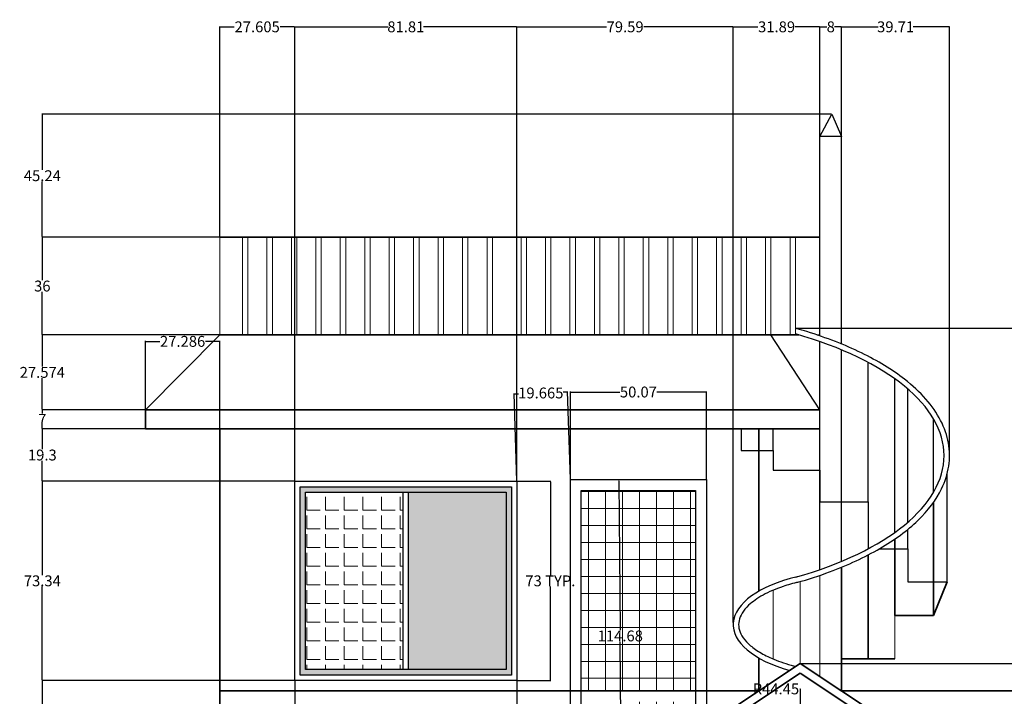
# Model space of a CAD drawing. Units: inches. Extents: x 1366 to 1929, y 372 to 1068.
# Tile 3 of 4: x 1366 to 1728, y 818 to 1068. Entities that reach past the tile are written whole.
import ezdxf

# ---------------------------------------------------------------- set-up
doc = ezdxf.new("R2010")
doc.units = ezdxf.units.IN
doc.header["$MEASUREMENT"] = 0
for name, color, linetype, lineweight in [('A-ANNO-DIMS', 2, 'Continuous', 18), ('A-DOOR', 4, 'Continuous', 30), ('A-ELEV', 7, 'Continuous', 35), ('A-ELEV-PATT', 252, 'Continuous', 13), ('A-ELEV-RAIL', 8, 'Continuous', 18), ('A-FLOR-STRS', 2, 'Continuous', 30), ('A-GLAZ', 4, 'Continuous', 30)]:
    doc.layers.add(name, color=color, linetype=linetype, lineweight=lineweight)
doc.styles.get("Standard").update_dxf_attribs({"font": 'arial.ttf'})
doc.dimstyles.get("Standard").update_dxf_attribs({"dimtxt": 4, "dimasz": 0.18, "dimexe": 0.18, "dimexo": 0.0625, "dimgap": 0.09, "dimtad": 0, "dimtih": 1, "dimtoh": 1, "dimdec": 0, "dimrnd": 6, "dimzin": 0, "dimdsep": 46, "dimlunit": 3, "dimtxsty": 'Standard', "dimcen": 0.09, "dimadec": 0, "dimazin": 0, "dimtfac": 1, "dimtdec": 0, "dimtofl": 0, "dimtmove": 0, "dimatfit": 3, "dimfxl": 1, "dimtolj": 1, "dimtzin": 0, "dimarcsym": 0})
pattern_1 = [(0, (0, 0), (0, 6.875), [5, -1.875]), (90, (0, 0), (-6.875, 4e-16), [5, -1.875])]

# ---------------------------------------------------------------- blocks, each defined once
blk = doc.blocks.new('WIN-750')
for p, q in [((4, 69.34), (77.81, 69.34)), ((4, 4), (4, 69.34)), ((77.81, 69.34), (77.81, 4)), ((77.81, 4), (4, 4))]:
    blk.add_line(p, q)
for points in [[(0, 73.34), (81.81, 73.34), (81.81, 0), (0, 0)], [(2, 71.34), (79.81, 71.34), (79.81, 2), (2, 2)]]:
    blk.add_lwpolyline(points, close=True)
blk = doc.blocks.new('*D4')
at = {"layer": 'A-ANNO-DIMS', "color": 0, "lineweight": -2, "transparency": 16777216}
for p, q in [((1466.83, 824.16), (1466.83, 811.78)), ((1548.64, 824.16), (1548.64, 811.78)), ((1467.01, 811.96), (1484.79, 811.96)), ((1548.46, 811.96), (1530.67, 811.96))]:
    blk.add_line(p, q, dxfattribs=at)
at = {"layer": 'A-ANNO-DIMS', "color": 0, "lineweight": 30, "transparency": 16777216}
for points in [[(1467.01, 811.99), (1467.01, 811.93), (1466.83, 811.96)], [(1548.46, 811.99), (1548.46, 811.93), (1548.64, 811.96)]]:
    blk.add_solid(points, dxfattribs=at)
at = {"layer": 'Defpoints', "color": 0, "lineweight": 30, "transparency": 16777216}
for p in [(1466.83, 824.23), (1548.64, 824.23), (1548.64, 811.96)]:
    blk.add_point(p, dxfattribs=at)
at = {"layer": 'A-ANNO-DIMS', "color": 0, "transparency": 16777216, "insert": (1507.73, 811.96), "char_height": 4, "attachment_point": 5}
blk.add_mtext('\\A1;WINDOW 82 TYP.', dxfattribs=at)
blk = doc.blocks.new('*D5')
at = {"layer": 'A-ANNO-DIMS', "color": 0, "lineweight": -2, "transparency": 16777216}
for p, q in [((1548.7, 897.57), (1561.09, 897.57)), ((1560.91, 897.39), (1560.91, 863.03)), ((1560.91, 824.41), (1560.91, 858.76)), ((1548.7, 824.23), (1561.09, 824.23))]:
    blk.add_line(p, q, dxfattribs=at)
at = {"layer": 'A-ANNO-DIMS', "color": 0, "lineweight": 30, "transparency": 16777216}
for points in [[(1560.88, 897.39), (1560.94, 897.39), (1560.91, 897.57)], [(1560.88, 824.41), (1560.94, 824.41), (1560.91, 824.23)]]:
    blk.add_solid(points, dxfattribs=at)
at = {"layer": 'Defpoints', "color": 0, "lineweight": 30, "transparency": 16777216}
for p in [(1548.64, 897.57), (1560.91, 897.57), (1548.64, 824.23)]:
    blk.add_point(p, dxfattribs=at)
at = {"layer": 'A-ANNO-DIMS', "color": 0, "transparency": 16777216, "insert": (1560.91, 860.9), "char_height": 4, "attachment_point": 5}
blk.add_mtext('\\A1;73 TYP.', dxfattribs=at)
blk = doc.blocks.new('*D10')
at = {"layer": 'A-ANNO-DIMS', "color": 0, "lineweight": -2, "transparency": 16777216}
for p, q in [((1439.22, 987.5), (1439.22, 1065.06)), ((1439.4, 1064.88), (1444.58, 1064.88)), ((1466.65, 1064.88), (1461.47, 1064.88)), ((1466.83, 897.63), (1466.83, 1065.06))]:
    blk.add_line(p, q, dxfattribs=at)
at = {"layer": 'A-ANNO-DIMS', "color": 0, "lineweight": 30, "transparency": 16777216}
for points in [[(1439.4, 1064.91), (1439.4, 1064.85), (1439.22, 1064.88)], [(1466.65, 1064.91), (1466.65, 1064.85), (1466.83, 1064.88)]]:
    blk.add_solid(points, dxfattribs=at)
at = {"layer": 'Defpoints', "color": 0, "lineweight": 30, "transparency": 16777216}
for p in [(1466.83, 1064.88), (1439.22, 987.44), (1466.83, 897.57)]:
    blk.add_point(p, dxfattribs=at)
at = {"layer": 'A-ANNO-DIMS', "color": 0, "transparency": 16777216, "insert": (1453.02, 1064.88), "char_height": 4, "attachment_point": 5}
blk.add_mtext('\\A1;27.605', dxfattribs=at)
blk = doc.blocks.new('*D11')
at = {"layer": 'A-ANNO-DIMS', "color": 0, "lineweight": -2, "transparency": 16777216}
for p, q in [((1466.83, 897.63), (1466.83, 1065.06)), ((1467.01, 1064.88), (1501.28, 1064.88)), ((1548.46, 1064.88), (1514.19, 1064.88)), ((1548.64, 897.63), (1548.64, 1065.06))]:
    blk.add_line(p, q, dxfattribs=at)
at = {"layer": 'A-ANNO-DIMS', "color": 0, "lineweight": 30, "transparency": 16777216}
for points in [[(1467.01, 1064.91), (1467.01, 1064.85), (1466.83, 1064.88)], [(1548.46, 1064.91), (1548.46, 1064.85), (1548.64, 1064.88)]]:
    blk.add_solid(points, dxfattribs=at)
at = {"layer": 'Defpoints', "color": 0, "lineweight": 30, "transparency": 16777216}
for p in [(1548.64, 1064.88), (1466.83, 897.57), (1548.64, 897.57)]:
    blk.add_point(p, dxfattribs=at)
at = {"layer": 'A-ANNO-DIMS', "color": 0, "transparency": 16777216, "insert": (1507.73, 1064.88), "char_height": 4, "attachment_point": 5}
blk.add_mtext('\\A1;81.81', dxfattribs=at)
blk = doc.blocks.new('*D12')
at = {"layer": 'A-ANNO-DIMS', "color": 0, "lineweight": -2, "transparency": 16777216}
for p, q in [((1548.64, 897.63), (1548.64, 1065.06)), ((1548.82, 1064.88), (1581.6, 1064.88)), ((1628.05, 1064.88), (1595.26, 1064.88)), ((1628.23, 845.55), (1628.23, 1065.06))]:
    blk.add_line(p, q, dxfattribs=at)
at = {"layer": 'A-ANNO-DIMS', "color": 0, "lineweight": 30, "transparency": 16777216}
for points in [[(1548.82, 1064.91), (1548.82, 1064.85), (1548.64, 1064.88)], [(1628.05, 1064.91), (1628.05, 1064.85), (1628.23, 1064.88)]]:
    blk.add_solid(points, dxfattribs=at)
at = {"layer": 'Defpoints', "color": 0, "lineweight": 30, "transparency": 16777216}
for p in [(1628.23, 1064.88), (1548.64, 897.57), (1628.23, 845.48)]:
    blk.add_point(p, dxfattribs=at)
at = {"layer": 'A-ANNO-DIMS', "color": 0, "transparency": 16777216, "insert": (1588.43, 1064.88), "char_height": 4, "attachment_point": 5}
blk.add_mtext('\\A1;79.59', dxfattribs=at)
blk = doc.blocks.new('*D13')
at = {"layer": 'A-ANNO-DIMS', "color": 0, "lineweight": -2, "transparency": 16777216}
for p, q in [((1628.23, 845.55), (1628.23, 1065.06)), ((1628.41, 1064.88), (1637.33, 1064.88)), ((1659.93, 1064.88), (1651.01, 1064.88)), ((1660.11, 1024.54), (1660.11, 1065.06))]:
    blk.add_line(p, q, dxfattribs=at)
at = {"layer": 'A-ANNO-DIMS', "color": 0, "lineweight": 30, "transparency": 16777216}
for points in [[(1628.41, 1064.91), (1628.41, 1064.85), (1628.23, 1064.88)], [(1659.93, 1064.91), (1659.93, 1064.85), (1660.11, 1064.88)]]:
    blk.add_solid(points, dxfattribs=at)
at = {"layer": 'Defpoints', "color": 0, "lineweight": 30, "transparency": 16777216}
for p in [(1660.11, 1064.88), (1660.11, 1024.48), (1628.23, 845.48)]:
    blk.add_point(p, dxfattribs=at)
at = {"layer": 'A-ANNO-DIMS', "color": 0, "transparency": 16777216, "insert": (1644.17, 1064.88), "char_height": 4, "attachment_point": 5}
blk.add_mtext('\\A1;31.89', dxfattribs=at)
blk = doc.blocks.new('*D14')
at = {"layer": 'A-ANNO-DIMS', "color": 0, "lineweight": -2, "transparency": 16777216}
for p, q in [((1660.11, 1024.54), (1660.11, 1065.06)), ((1660.29, 1064.88), (1662.71, 1064.88)), ((1667.93, 1064.88), (1665.52, 1064.88)), ((1668.11, 1024.54), (1668.11, 1065.06))]:
    blk.add_line(p, q, dxfattribs=at)
at = {"layer": 'A-ANNO-DIMS', "color": 0, "lineweight": 30, "transparency": 16777216}
for points in [[(1660.29, 1064.91), (1660.29, 1064.85), (1660.11, 1064.88)], [(1667.93, 1064.91), (1667.93, 1064.85), (1668.11, 1064.88)]]:
    blk.add_solid(points, dxfattribs=at)
at = {"layer": 'Defpoints', "color": 0, "lineweight": 30, "transparency": 16777216}
for p in [(1668.11, 1064.88), (1660.11, 1024.48), (1668.11, 1024.48)]:
    blk.add_point(p, dxfattribs=at)
at = {"layer": 'A-ANNO-DIMS', "color": 0, "transparency": 16777216, "insert": (1664.11, 1064.88), "char_height": 4, "attachment_point": 5}
blk.add_mtext('\\A1;8', dxfattribs=at)
blk = doc.blocks.new('*D15')
at = {"layer": 'A-ANNO-DIMS', "color": 0, "lineweight": -2, "transparency": 16777216}
for p, q in [((1668.11, 1024.54), (1668.11, 1065.06)), ((1668.29, 1064.88), (1681.52, 1064.88)), ((1707.64, 1064.88), (1694.42, 1064.88)), ((1707.82, 907.44), (1707.82, 1065.06))]:
    blk.add_line(p, q, dxfattribs=at)
at = {"layer": 'A-ANNO-DIMS', "color": 0, "lineweight": 30, "transparency": 16777216}
for points in [[(1668.29, 1064.91), (1668.29, 1064.85), (1668.11, 1064.88)], [(1707.64, 1064.91), (1707.64, 1064.85), (1707.82, 1064.88)]]:
    blk.add_solid(points, dxfattribs=at)
at = {"layer": 'Defpoints', "color": 0, "lineweight": 30, "transparency": 16777216}
for p in [(1707.82, 1064.88), (1668.11, 1024.48), (1707.82, 907.38)]:
    blk.add_point(p, dxfattribs=at)
at = {"layer": 'A-ANNO-DIMS', "color": 0, "transparency": 16777216, "insert": (1687.97, 1064.88), "char_height": 4, "attachment_point": 5}
blk.add_mtext('\\A1;39.71', dxfattribs=at)
blk = doc.blocks.new('*D36')
at = {"layer": 'A-ANNO-DIMS', "color": 0, "lineweight": -2, "transparency": 16777216}
for p, q in [((1466.76, 824.23), (1373.77, 824.23)), ((1373.95, 824.05), (1373.95, 804.44)), ((1373.95, 780.56), (1373.95, 800.17)), ((1439.16, 780.38), (1373.77, 780.38))]:
    blk.add_line(p, q, dxfattribs=at)
at = {"layer": 'A-ANNO-DIMS', "color": 0, "lineweight": 30, "transparency": 16777216}
for points in [[(1373.92, 824.05), (1373.98, 824.05), (1373.95, 824.23)], [(1373.92, 780.56), (1373.98, 780.56), (1373.95, 780.38)]]:
    blk.add_solid(points, dxfattribs=at)
at = {"layer": 'Defpoints', "color": 0, "lineweight": 30, "transparency": 16777216}
for p in [(1373.95, 824.23), (1466.83, 824.23), (1439.22, 780.38)]:
    blk.add_point(p, dxfattribs=at)
at = {"layer": 'A-ANNO-DIMS', "color": 0, "transparency": 16777216, "insert": (1373.95, 802.3), "char_height": 4, "attachment_point": 5}
blk.add_mtext('\\A1;43.85', dxfattribs=at)
blk = doc.blocks.new('*D37')
at = {"layer": 'A-ANNO-DIMS', "color": 0, "lineweight": -2, "transparency": 16777216}
for p, q in [((1466.76, 897.57), (1373.77, 897.57)), ((1373.95, 897.39), (1373.95, 863.03)), ((1373.95, 824.41), (1373.95, 858.76)), ((1466.76, 824.23), (1373.77, 824.23))]:
    blk.add_line(p, q, dxfattribs=at)
at = {"layer": 'A-ANNO-DIMS', "color": 0, "lineweight": 30, "transparency": 16777216}
for points in [[(1373.92, 897.39), (1373.98, 897.39), (1373.95, 897.57)], [(1373.92, 824.41), (1373.98, 824.41), (1373.95, 824.23)]]:
    blk.add_solid(points, dxfattribs=at)
at = {"layer": 'Defpoints', "color": 0, "lineweight": 30, "transparency": 16777216}
for p in [(1373.95, 897.57), (1466.83, 897.57), (1466.83, 824.23)]:
    blk.add_point(p, dxfattribs=at)
at = {"layer": 'A-ANNO-DIMS', "color": 0, "transparency": 16777216, "insert": (1373.95, 860.9), "char_height": 4, "attachment_point": 5}
blk.add_mtext('\\A1;73.34', dxfattribs=at)
blk = doc.blocks.new('*D38')
at = {"layer": 'A-ANNO-DIMS', "color": 0, "lineweight": -2, "transparency": 16777216}
for p, q in [((1439.16, 916.87), (1373.77, 916.87)), ((1373.95, 916.69), (1373.95, 909.35)), ((1373.95, 897.75), (1373.95, 905.08)), ((1466.76, 897.57), (1373.77, 897.57))]:
    blk.add_line(p, q, dxfattribs=at)
at = {"layer": 'A-ANNO-DIMS', "color": 0, "lineweight": 30, "transparency": 16777216}
for points in [[(1373.92, 916.69), (1373.98, 916.69), (1373.95, 916.87)], [(1373.92, 897.75), (1373.98, 897.75), (1373.95, 897.57)]]:
    blk.add_solid(points, dxfattribs=at)
at = {"layer": 'Defpoints', "color": 0, "lineweight": 30, "transparency": 16777216}
for p in [(1373.95, 916.87), (1439.22, 916.87), (1466.83, 897.57)]:
    blk.add_point(p, dxfattribs=at)
at = {"layer": 'A-ANNO-DIMS', "color": 0, "transparency": 16777216, "insert": (1373.95, 907.22), "char_height": 4, "attachment_point": 5}
blk.add_mtext('\\A1;19.3', dxfattribs=at)
blk = doc.blocks.new('*D39')
at = {"layer": 'A-ANNO-DIMS', "color": 0, "lineweight": -2, "transparency": 16777216}
for p, q in [((1411.87353, 923.866592), (1373.772656, 923.866592)), ((1373.952656, 923.686592), (1373.952656, 922.456592)), ((1439.159301, 916.866592), (1373.772656, 916.866592)), ((1373.952656, 917.046592), (1373.952656, 918.276592))]:
    blk.add_line(p, q, dxfattribs=at)
at = {"layer": 'A-ANNO-DIMS', "color": 0, "lineweight": 30, "transparency": 16777216}
for points in [[(1373.922656, 923.686592), (1373.982656, 923.686592), (1373.952656, 923.866592)], [(1373.922656, 917.046592), (1373.982656, 917.046592), (1373.952656, 916.866592)]]:
    blk.add_solid(points, dxfattribs=at)
at = {"layer": 'Defpoints', "color": 0, "lineweight": 30, "transparency": 16777216}
for p in [(1373.952656, 923.866592), (1411.93603, 923.866592), (1439.221801, 916.866592)]:
    blk.add_point(p, dxfattribs=at)
at = {"layer": 'A-ANNO-DIMS', "color": 0, "transparency": 16777216, "insert": (1373.952656, 920.366592), "char_height": 4, "attachment_point": 5}
blk.add_mtext('\\A1;7', dxfattribs=at)
blk = doc.blocks.new('*D40')
at = {"layer": 'A-ANNO-DIMS', "color": 0, "lineweight": -2, "transparency": 16777216}
for p, q in [((1439.16, 951.44), (1373.77, 951.44)), ((1373.95, 951.26), (1373.95, 939.79)), ((1373.95, 924.05), (1373.95, 935.52)), ((1411.87, 923.87), (1373.77, 923.87))]:
    blk.add_line(p, q, dxfattribs=at)
at = {"layer": 'A-ANNO-DIMS', "color": 0, "lineweight": 30, "transparency": 16777216}
for points in [[(1373.92, 951.26), (1373.98, 951.26), (1373.95, 951.44)], [(1373.92, 924.05), (1373.98, 924.05), (1373.95, 923.87)]]:
    blk.add_solid(points, dxfattribs=at)
at = {"layer": 'Defpoints', "color": 0, "lineweight": 30, "transparency": 16777216}
for p in [(1373.95, 951.44), (1439.22, 951.44), (1411.94, 923.87)]:
    blk.add_point(p, dxfattribs=at)
at = {"layer": 'A-ANNO-DIMS', "color": 0, "transparency": 16777216, "insert": (1373.95, 937.65), "char_height": 4, "attachment_point": 5}
blk.add_mtext('\\A1;27.574', dxfattribs=at)
blk = doc.blocks.new('*D41')
at = {"layer": 'A-ANNO-DIMS', "color": 0, "lineweight": -2, "transparency": 16777216}
for p, q in [((1439.16, 987.44), (1373.77, 987.44)), ((1373.95, 987.26), (1373.95, 971.57)), ((1373.95, 951.62), (1373.95, 967.31)), ((1439.16, 951.44), (1373.77, 951.44))]:
    blk.add_line(p, q, dxfattribs=at)
at = {"layer": 'A-ANNO-DIMS', "color": 0, "lineweight": 30, "transparency": 16777216}
for points in [[(1373.92, 987.26), (1373.98, 987.26), (1373.95, 987.44)], [(1373.92, 951.62), (1373.98, 951.62), (1373.95, 951.44)]]:
    blk.add_solid(points, dxfattribs=at)
at = {"layer": 'Defpoints', "color": 0, "lineweight": 30, "transparency": 16777216}
for p in [(1373.95, 987.44), (1439.22, 987.44), (1439.22, 951.44)]:
    blk.add_point(p, dxfattribs=at)
at = {"layer": 'A-ANNO-DIMS', "color": 0, "transparency": 16777216, "insert": (1373.95, 969.44), "char_height": 4, "attachment_point": 5}
blk.add_mtext('\\A1;36', dxfattribs=at)
blk = doc.blocks.new('*D42')
at = {"layer": 'A-ANNO-DIMS', "color": 0, "lineweight": -2, "transparency": 16777216}
for p, q in [((1664.41, 1032.68), (1373.77, 1032.68)), ((1373.95, 1032.5), (1373.95, 1012.19)), ((1373.95, 987.62), (1373.95, 1007.93)), ((1439.16, 987.44), (1373.77, 987.44))]:
    blk.add_line(p, q, dxfattribs=at)
at = {"layer": 'A-ANNO-DIMS', "color": 0, "lineweight": 30, "transparency": 16777216}
for points in [[(1373.92, 1032.5), (1373.98, 1032.5), (1373.95, 1032.68)], [(1373.92, 987.62), (1373.98, 987.62), (1373.95, 987.44)]]:
    blk.add_solid(points, dxfattribs=at)
at = {"layer": 'Defpoints', "color": 0, "lineweight": 30, "transparency": 16777216}
for p in [(1373.95, 1032.68), (1664.48, 1032.68), (1439.22, 987.44)]:
    blk.add_point(p, dxfattribs=at)
at = {"layer": 'A-ANNO-DIMS', "color": 0, "transparency": 16777216, "insert": (1373.95, 1010.06), "char_height": 4, "attachment_point": 5}
blk.add_mtext('\\A1;45.24', dxfattribs=at)
blk = doc.blocks.new('*D49')
at = {"layer": 'A-ANNO-DIMS', "color": 0, "lineweight": -2, "transparency": 16777216}
for p, q in [((1652.94, 830.47), (1920.61, 830.47)), ((1920.43, 830.29), (1920.43, 827.56)), ((1920.43, 820.56), (1920.43, 823.29)), ((1861, 820.38), (1920.61, 820.38))]:
    blk.add_line(p, q, dxfattribs=at)
at = {"layer": 'A-ANNO-DIMS', "color": 0, "lineweight": 30, "transparency": 16777216}
for points in [[(1920.4, 830.29), (1920.46, 830.29), (1920.43, 830.47)], [(1920.4, 820.56), (1920.46, 820.56), (1920.43, 820.38)]]:
    blk.add_solid(points, dxfattribs=at)
at = {"layer": 'Defpoints', "color": 0, "lineweight": 30, "transparency": 16777216}
for p in [(1652.88, 830.47), (1920.43, 830.47), (1860.94, 820.38)]:
    blk.add_point(p, dxfattribs=at)
at = {"layer": 'A-ANNO-DIMS', "color": 0, "transparency": 16777216, "insert": (1920.43, 825.42), "char_height": 4, "attachment_point": 5}
blk.add_mtext('\\A1;10.089', dxfattribs=at)
blk = doc.blocks.new('*D50')
at = {"layer": 'A-ANNO-DIMS', "color": 0, "lineweight": -2, "transparency": 16777216}
for p, q in [((1651.18, 953.9), (1920.61, 953.9)), ((1920.43, 953.72), (1920.43, 894.32)), ((1920.43, 830.65), (1920.43, 890.05)), ((1652.94, 830.47), (1920.61, 830.47))]:
    blk.add_line(p, q, dxfattribs=at)
at = {"layer": 'A-ANNO-DIMS', "color": 0, "lineweight": 30, "transparency": 16777216}
for points in [[(1920.4, 953.72), (1920.46, 953.72), (1920.43, 953.9)], [(1920.4, 830.65), (1920.46, 830.65), (1920.43, 830.47)]]:
    blk.add_solid(points, dxfattribs=at)
at = {"layer": 'Defpoints', "color": 0, "lineweight": 30, "transparency": 16777216}
for p in [(1651.11, 953.9), (1920.43, 953.9), (1652.88, 830.47)]:
    blk.add_point(p, dxfattribs=at)
at = {"layer": 'A-ANNO-DIMS', "color": 0, "transparency": 16777216, "insert": (1920.43, 892.18), "char_height": 4, "attachment_point": 5}
blk.add_mtext('\\A1;123.43', dxfattribs=at)
blk = doc.blocks.new('*D52')
at = {"layer": 'A-ANNO-DIMS', "color": 0, "lineweight": -2, "transparency": 16777216}
for p, q in [((1568.29, 898.28), (1568.29, 930.6)), ((1568.47, 930.42), (1586.49, 930.42)), ((1618.18, 930.42), (1600.16, 930.42)), ((1618.36, 898.28), (1618.36, 930.6))]:
    blk.add_line(p, q, dxfattribs=at)
at = {"layer": 'A-ANNO-DIMS', "color": 0, "lineweight": 30, "transparency": 16777216}
for points in [[(1568.47, 930.45), (1568.47, 930.39), (1568.29, 930.42)], [(1618.18, 930.45), (1618.18, 930.39), (1618.36, 930.42)]]:
    blk.add_solid(points, dxfattribs=at)
at = {"layer": 'Defpoints', "color": 0, "lineweight": 30, "transparency": 16777216}
for p in [(1618.36, 930.42), (1568.29, 898.22), (1618.36, 898.22)]:
    blk.add_point(p, dxfattribs=at)
at = {"layer": 'A-ANNO-DIMS', "color": 0, "transparency": 16777216, "insert": (1593.32, 930.42), "char_height": 4, "attachment_point": 5}
blk.add_mtext('\\A1;50.07', dxfattribs=at)
blk = doc.blocks.new('*D53')
at = {"layer": 'A-ANNO-DIMS', "color": 0, "lineweight": -2, "transparency": 16777216}
for p, q in [((1548.63, 897.63), (1547.56, 929.93)), ((1547.75, 929.75), (1549.18, 929.8)), ((1567.04, 930.39), (1565.61, 930.35)), ((1568.29, 898.28), (1567.22, 930.58))]:
    blk.add_line(p, q, dxfattribs=at)
at = {"layer": 'A-ANNO-DIMS', "color": 0, "lineweight": 30, "transparency": 16777216}
for points in [[(1547.75, 929.78), (1547.75, 929.72), (1547.57, 929.75)], [(1567.04, 930.42), (1567.04, 930.36), (1567.22, 930.4)]]:
    blk.add_solid(points, dxfattribs=at)
at = {"layer": 'Defpoints', "color": 0, "lineweight": 30, "transparency": 16777216}
for p in [(1567.22, 930.4), (1548.64, 897.57), (1568.29, 898.22)]:
    blk.add_point(p, dxfattribs=at)
at = {"layer": 'A-ANNO-DIMS', "color": 0, "transparency": 16777216, "insert": (1557.4, 930.07), "char_height": 4, "attachment_point": 5}
blk.add_mtext('\\A1;19.665', dxfattribs=at)
blk = doc.blocks.new('*D56')
at = {"layer": 'A-ANNO-DIMS', "color": 0, "lineweight": -2, "transparency": 16777216}
for p, q in [((1411.94, 916.93), (1411.94, 949.25)), ((1412.12, 949.07), (1417.15, 949.07)), ((1439.04, 949.07), (1434, 949.07)), ((1439.22, 916.93), (1439.22, 949.25))]:
    blk.add_line(p, q, dxfattribs=at)
at = {"layer": 'A-ANNO-DIMS', "color": 0, "lineweight": 30, "transparency": 16777216}
for points in [[(1412.12, 949.1), (1412.12, 949.04), (1411.94, 949.07)], [(1439.04, 949.1), (1439.04, 949.04), (1439.22, 949.07)]]:
    blk.add_solid(points, dxfattribs=at)
at = {"layer": 'Defpoints', "color": 0, "lineweight": 30, "transparency": 16777216}
for p in [(1439.22, 949.07), (1411.94, 916.87), (1439.22, 916.87)]:
    blk.add_point(p, dxfattribs=at)
at = {"layer": 'A-ANNO-DIMS', "color": 0, "transparency": 16777216, "insert": (1425.58, 949.07), "char_height": 4, "attachment_point": 5}
blk.add_mtext('\\A1;27.286', dxfattribs=at)
blk = doc.blocks.new('*D57')
at = {"layer": 'A-ANNO-DIMS', "color": 0, "lineweight": -2, "transparency": 16777216}
for p, q in [((1618.3, 898.22), (1585.98, 897.94)), ((1586.16, 897.77), (1586.63, 842.74)), ((1587.13, 783.45), (1586.66, 838.48)), ((1619.27, 783.54), (1586.95, 783.27))]:
    blk.add_line(p, q, dxfattribs=at)
at = {"layer": 'A-ANNO-DIMS', "color": 0, "lineweight": 30, "transparency": 16777216}
for points in [[(1586.19, 897.77), (1586.13, 897.77), (1586.16, 897.95)], [(1587.16, 783.45), (1587.1, 783.45), (1587.13, 783.27)]]:
    blk.add_solid(points, dxfattribs=at)
at = {"layer": 'Defpoints', "color": 0, "lineweight": 30, "transparency": 16777216}
for p in [(1586.16, 897.95), (1618.36, 898.22), (1619.33, 783.54)]:
    blk.add_point(p, dxfattribs=at)
at = {"layer": 'A-ANNO-DIMS', "color": 0, "transparency": 16777216, "insert": (1586.65, 840.61), "char_height": 4, "attachment_point": 5}
blk.add_mtext('\\A1;114.68', dxfattribs=at)
blk = doc.blocks.new('*D65')
at = {"layer": 'A-ANNO-DIMS', "color": 0, "lineweight": -2, "transparency": 16777216}
for p, q in [((1652.7, 821.11), (1652.88, 821.11)), ((1652.88, 821.11), (1652.88, 794.62)), ((1652.88, 749.9), (1652.88, 750.08)), ((1652.79, 749.99), (1652.97, 749.99))]:
    blk.add_line(p, q, dxfattribs=at)
at = {"layer": 'A-ANNO-DIMS', "color": 0, "lineweight": 30, "transparency": 16777216}
blk.add_solid([(1652.91, 794.62), (1652.85, 794.62), (1652.88, 794.44)], dxfattribs=at)
at = {"layer": 'Defpoints', "color": 0, "lineweight": 30, "transparency": 16777216}
for p in [(1652.88, 794.44), (1652.88, 749.99)]:
    blk.add_point(p, dxfattribs=at)
at = {"layer": 'A-ANNO-DIMS', "color": 0, "transparency": 16777216, "insert": (1643.93, 821.11), "char_height": 4, "attachment_point": 5}
blk.add_mtext('\\A1;R44.45', dxfattribs=at)

msp = doc.modelspace()

# ---------------------------------------------------------------- hatches: boundary and pattern name
at = {"layer": 'A-ELEV-PATT'}
h = msp.add_hatch(color=256, dxfattribs=at)
h.dxf.hatch_style = 1
h.paths.add_polyline_path([(1546.6356, 729.6227), (1468.827, 729.6227), (1468.827, 660.2826), (1546.6356, 660.2826)])
h.paths.add_polyline_path([(1544.6356, 662.2826), (1470.827, 662.2826), (1470.827, 727.6227), (1544.6356, 727.6227)], flags=16)
h.paths.add_polyline_path([(1818.7172, 725.6227), (1748.9085, 725.6227), (1748.9085, 664.2826), (1818.7172, 664.2826)])
h.paths.add_polyline_path([(1750.9085, 723.6227), (1816.7172, 723.6227), (1816.7172, 666.2826), (1750.9085, 666.2826)], flags=16)
h.paths.add_polyline_path([(1546.6356, 895.5665), (1468.827, 895.5665), (1468.827, 826.2264), (1546.6356, 826.2264)])
h.paths.add_polyline_path([(1544.6356, 828.2264), (1470.827, 828.2264), (1470.827, 893.5665), (1544.6356, 893.5665)], flags=16)
h = msp.add_hatch(dxfattribs=at)
h.set_pattern_fill('ANGLE', color=256, scale=25)
h.set_pattern_definition(pattern_1)
h.paths.add_polyline_path([(1506.6356, 893.5665), (1470.827, 893.5665), (1470.827, 828.2264), (1506.6356, 828.2264)])
h = msp.add_hatch(dxfattribs=at)
h.set_pattern_fill('ANGLE', color=256, scale=25)
h.set_pattern_definition(pattern_1)
h.paths.add_polyline_path([(1544.6356, 893.5665), (1508.6356, 893.5665), (1508.6356, 828.2264), (1544.6356, 828.2264)])
h.paths.add_polyline_path([(1506.6356, 727.6227), (1470.827, 727.6227), (1470.827, 662.2826), (1506.6356, 662.2826)])
h.paths.add_polyline_path([(1544.6356, 727.6227), (1508.6356, 727.6227), (1508.6356, 662.2826), (1544.6356, 662.2826)])
h.paths.add_polyline_path([(1608.5338, 752.9927), (1697.2248, 752.9927, 0.93463511)])
h.paths.add_polyline_path([(1682.8585, 567.593), (1622.7881, 567.593), (1622.7881, 535.593), (1682.8585, 535.593)])
h.paths.add_polyline_path([(1782.7172, 723.6227), (1750.9085, 723.6227), (1750.9085, 666.2826), (1782.7172, 666.2826)])
h.paths.add_polyline_path([(1816.7172, 723.6227), (1784.7172, 723.6227), (1784.7172, 666.2826), (1816.7172, 666.2826)])
h.paths.add_polyline_path([(1817.1901, 526.1862), (1739.2847, 526.1862), (1739.2847, 513.1136), (1817.1901, 513.1136)])
h.paths.add_polyline_path([(1565.633, 526.1862), (1487.7276, 526.1862), (1487.7276, 513.1136), (1565.633, 513.1136)])
h = msp.add_hatch(dxfattribs=at)
h.set_pattern_fill('NET', color=256, scale=50)
h.paths.add_polyline_path([(1614.2855, 894.2183), (1572.2896, 894.2183), (1572.2896, 889.0571), (1572.2896, 820.3796), (1614.2855, 820.3796)])
h.paths.add_polyline_path([(1579.6001, 816.3796), (1575.6001, 816.3796), (1575.6001, 786.5447), (1579.6001, 786.5447)])
h.paths.add_polyline_path([(1585.6001, 816.3796), (1581.6001, 816.3796), (1581.6001, 786.5447), (1585.6001, 786.5447)])
h.paths.add_polyline_path([(1591.6001, 816.3796), (1587.6001, 816.3796), (1587.6001, 787.3399), (1591.6001, 789.9826)])
h.paths.add_polyline_path([(1600.6001, 816.3796), (1593.6001, 816.3796), (1593.6001, 791.3039), (1600.6001, 795.9287)])
h.paths.add_polyline_path([(1609.6001, 816.3796), (1602.6001, 816.3796), (1602.6001, 797.2501), (1609.6001, 801.8748)])
h.paths.add_polyline_path([(1573.6001, 816.3796), (1572.2896, 816.3796), (1572.2896, 786.5447), (1573.6001, 786.5447)])

# ---------------------------------------------------------------- linework, layer by layer
at = {"layer": 'A-DOOR'}
for p, q in [((1568.2896, 889.0571), (1568.2896, 898.2183)), ((1568.2896, 898.2183), (1618.3601, 898.2183)), ((1618.3601, 898.2183), (1618.3601, 807.6624)), ((1572.2896, 889.0571), (1572.2896, 894.2183)), ((1572.2896, 894.2183), (1614.2855, 894.2183)), ((1614.2855, 894.2183), (1614.2855, 820.3796)), ((1568.2896, 782.5447), (1568.2896, 889.0571)), ((1572.2896, 786.5447), (1572.2896, 889.0571)), ((1614.3601, 820.3796), (1614.3601, 805.0197))]:
    msp.add_line(p, q, dxfattribs=at)
at = {"layer": 'A-ELEV'}
for p, q in [((1439.2218, 987.441), (1660.1133, 987.441)), ((1439.2218, 951.441), (1411.936, 923.8666)), ((1439.2218, 951.441), (1652.4124, 951.441)), ((1660.1133, 923.8666), (1411.936, 923.8666)), ((1411.936, 923.8666), (1411.936, 916.8666)), ((1439.2218, 916.8666), (1411.936, 916.8666)), ((1439.2218, 780.3796), (1439.2218, 916.8666)), ((1439.2218, 916.8666), (1660.1133, 916.8666)), ((1439.2218, 780.3796), (1439.2218, 916.8666)), ((1637.6087, 857.0443), (1637.6087, 916.8666)), ((1701.9119, 848.1865), (1701.9119, 889.7659)), ((1687.7189, 848.1865), (1687.7189, 876.3021)), ((1677.893, 870.4458), (1677.893, 832.1871)), ((1668.1133, 820.3796), (1668.1133, 865.9323)), ((1707.0068, 860.5497), (1701.9119, 848.1865)), ((1701.9119, 848.1865), (1687.7189, 848.1865)), ((1652.8793, 830.4686), (1547.7212, 760.9927)), ((1637.6087, 820.3796), (1637.6087, 832.5116)), ((1652.8793, 830.4686), (1757.7853, 760.9927)), ((1687.7189, 832.1871), (1668.1133, 832.1871)), ((1652.8773, 826.8716), (1551.8874, 760.1496)), ((1652.8773, 826.8716), (1753.6243, 760.1501)), ((1439.2218, 820.3796), (1637.6087, 820.3796)), ((1668.1133, 820.3796), (1860.9351, 820.3796))]:
    msp.add_line(p, q, dxfattribs=at)
at = {"layer": 'A-ELEV-RAIL'}
for p, q in [((1439.2218, 951.441), (1439.2218, 987.441)), ((1447.6001, 987.441), (1447.6001, 951.441)), ((1449.6001, 987.441), (1449.6001, 951.441)), ((1456.6001, 987.441), (1456.6001, 951.441)), ((1458.6001, 987.441), (1458.6001, 951.441)), ((1465.6001, 987.441), (1465.6001, 951.441)), ((1467.6001, 987.441), (1467.6001, 951.441)), ((1474.6001, 987.441), (1474.6001, 951.441)), ((1476.6001, 987.441), (1476.6001, 951.441)), ((1483.6001, 987.441), (1483.6001, 951.441)), ((1485.6001, 987.441), (1485.6001, 951.441)), ((1492.6001, 987.441), (1492.6001, 951.441)), ((1494.6001, 987.441), (1494.6001, 951.441)), ((1501.6001, 987.441), (1501.6001, 951.441)), ((1503.6001, 987.441), (1503.6001, 951.441)), ((1510.6001, 987.441), (1510.6001, 951.441)), ((1512.6001, 987.441), (1512.6001, 951.441)), ((1519.6001, 987.441), (1519.6001, 951.441)), ((1521.6001, 987.441), (1521.6001, 951.441)), ((1528.6001, 987.441), (1528.6001, 951.441)), ((1530.6001, 987.441), (1530.6001, 951.441)), ((1537.6001, 987.441), (1537.6001, 951.441)), ((1539.6001, 987.441), (1539.6001, 951.441)), ((1550.1133, 987.441), (1550.1133, 951.441)), ((1552.1133, 987.441), (1552.1133, 951.441)), ((1559.1133, 987.441), (1559.1133, 951.441)), ((1561.1133, 987.441), (1561.1133, 951.441)), ((1568.1133, 987.441), (1568.1133, 951.441)), ((1570.1133, 987.441), (1570.1133, 951.441)), ((1577.1133, 987.441), (1577.1133, 951.441)), ((1579.1133, 987.441), (1579.1133, 951.441)), ((1586.1133, 987.441), (1586.1133, 951.441)), ((1588.1133, 987.441), (1588.1133, 951.441)), ((1595.1133, 987.441), (1595.1133, 951.441)), ((1597.1133, 987.441), (1597.1133, 951.441)), ((1604.1133, 987.441), (1604.1133, 951.441)), ((1606.1133, 987.441), (1606.1133, 951.441)), ((1613.1133, 987.441), (1613.1133, 951.441)), ((1615.1133, 987.441), (1615.1133, 951.441)), ((1622.1133, 987.441), (1622.1133, 951.441)), ((1624.1133, 987.441), (1624.1133, 951.441)), ((1631.1133, 987.441), (1631.1133, 951.441)), ((1633.1133, 987.441), (1633.1133, 951.441)), ((1640.1133, 987.441), (1640.1133, 951.441)), ((1642.1133, 987.441), (1642.1133, 951.441)), ((1649.1133, 987.441), (1649.1133, 951.441)), ((1651.1133, 987.441), (1651.1133, 951.441)), ((1660.1133, 825.6777), (1660.1133, 862.924)), ((1652.8793, 860.6224), (1652.8793, 830.4686)), ((1642.9566, 857.4502), (1642.9566, 832.1053)), ((1687.7189, 848.1865), (1687.7189, 832.1871))]:
    msp.add_line(p, q, dxfattribs=at)
at = {"layer": 'A-FLOR-STRS'}
for p, q in [((1660.1133, 1024.4825), (1664.476, 1032.684)), ((1664.476, 1032.684), (1668.1133, 1024.4825)), ((1668.1133, 1024.4825), (1660.1133, 1024.4825)), ((1660.1133, 951.0866), (1660.1133, 1024.4825)), ((1668.1133, 948.0784), (1668.1133, 1024.4825)), ((1660.1133, 923.8666), (1642.1133, 951.441)), ((1659.0711, 951.441), (1660.1133, 951.441)), ((1660.1133, 865.0406), (1660.1133, 948.9702)), ((1668.1133, 868.0969), (1668.1133, 945.9139)), ((1677.893, 890.0032), (1677.893, 941.3061)), ((1687.7189, 878.745), (1687.7189, 935.2658)), ((1692.4499, 882.454), (1692.4499, 931.5568)), ((1701.9119, 893.4461), (1701.9119, 920.5647)), ((1631.1133, 916.8666), (1631.1133, 908.9116)), ((1642.9566, 908.9116), (1642.9566, 916.8666)), ((1631.1133, 908.9116), (1642.9566, 908.9116)), ((1642.9566, 908.9116), (1642.9566, 901.6391)), ((1642.9566, 901.6391), (1660.1133, 901.6391)), ((1660.1133, 901.6391), (1660.1133, 890.0032)), ((1707.0068, 860.5497), (1707.0068, 900.51)), ((1660.1133, 890.0032), (1677.893, 890.0032)), ((1677.893, 890.0032), (1677.893, 872.7047)), ((1692.4499, 872.7047), (1692.4499, 879.8433)), ((1682.0147, 872.7047), (1692.4499, 872.7047)), ((1692.4499, 872.7047), (1692.4499, 860.5497)), ((1692.4499, 860.5497), (1707.0068, 860.5497))]:
    msp.add_line(p, q, dxfattribs=at)
for centre, major_axis, ratio, start_param, end_param in [((1587.7373, 907.0054), (-118.088, 0), 0.44974202, 2.13721551, 4.1459698), ((1672.6941, 844.778), (-44.4966, 0), 0.44821311, 5.20331697, 7.29218917)]:
    msp.add_ellipse(centre, major_axis=major_axis, ratio=ratio, start_param=start_param, end_param=end_param, dxfattribs=at)
for points, knots in [([(1651.655, 860.2675), (1655.8372, 861.4637), (1659.8577, 862.7782), (1670.5016, 866.7365), (1676.7074, 869.6178), (1687.61, 875.9587), (1692.3075, 879.4178), (1699.963, 886.796), (1702.9233, 890.7181), (1706.2273, 897.5231), (1707.1131, 900.3162), (1707.9588, 905.9588), (1707.9171, 908.8066), (1706.9082, 914.4391), (1705.9425, 917.2222), (1703.1465, 922.6397), (1701.3172, 925.275), (1696.8618, 930.3542), (1694.2353, 932.7987), (1686.7428, 938.6372), (1681.4129, 941.8896), (1669.3457, 947.7682), (1662.6083, 950.3937), (1654.1168, 953.0248), (1652.893, 953.3892), (1651.655, 953.7433), (1651.4747, 953.7948), (1651.2941, 953.8462), (1651.1133, 953.8973)], [2.13721551, 2.13721551, 2.13721551, 2.13721551, 2.26172506, 2.26172506, 2.48335181, 2.48335181, 2.70497856, 2.70497856, 2.92660531, 2.92660531, 3.07429372, 3.07429372, 3.22198213, 3.22198213, 3.36967054, 3.36967054, 3.51735895, 3.51735895, 3.66504736, 3.66504736, 3.8870803, 3.8870803, 4.10911324, 4.10911324, 4.1459698, 4.1459698, 4.1459698, 4.15133644, 4.15133644, 4.15133644, 4.15133644]), ([(1652.1824, 860.4215), (1650.2195, 859.9512), (1648.3427, 859.414), (1643.8223, 857.8892), (1641.3375, 856.8165), (1637.0653, 854.4734), (1635.2796, 853.2027), (1632.8768, 850.9426), (1632.0756, 849.9691), (1630.9019, 848.0514), (1630.528, 847.11), (1630.1535, 845.2665), (1630.1489, 844.3614), (1630.5038, 842.5195), (1630.8671, 841.5795), (1632.0185, 839.6633), (1632.8081, 838.6899), (1634.8225, 836.7722), (1636.0465, 835.8289), (1638.8926, 834.0306), (1640.5141, 833.1755), (1644.4841, 831.4262), (1646.9138, 830.5633), (1649.5336, 829.8242), (1650.0872, 829.668), (1650.6493, 829.5174), (1651.2199, 829.3722)], [5.20331697, 5.20331697, 5.20331697, 5.20331697, 5.3575496, 5.3575496, 5.59802147, 5.59802147, 5.83849335, 5.83849335, 6.0154381, 6.0154381, 6.19238286, 6.19238286, 6.36932762, 6.36932762, 6.54627237, 6.54627237, 6.72321713, 6.72321713, 6.90016189, 6.90016189, 7.07710664, 7.07710664, 7.29218917, 7.29218917, 7.29218917, 7.33763881, 7.33763881, 7.33763881, 7.33763881])]:
    msp.add_open_spline(points, degree=3, knots=knots, dxfattribs=at)
at = {"layer": 'A-GLAZ'}
for p, q in [((1506.6356, 893.5665), (1506.6356, 828.2264)), ((1508.6356, 893.5665), (1508.6356, 828.2264))]:
    msp.add_line(p, q, dxfattribs=at)

# ---------------------------------------------------------------- block references
msp.add_blockref('WIN-750', (1466.827, 824.2268), dxfattribs=at)

# ---------------------------------------------------------------- dimensions: what is measured, and where the dimension line sits
at = {"layer": 'A-ANNO-DIMS'}
for base, p1, p2, override, picture, middle in [((1466.827, 1064.884), (1439.2218, 987.441), (1466.827, 897.5665), {"dimdec": 3, "dimlfac": 1, "dimrnd": 0, "dimzin": 0, "dimdsep": 46, "dimlunit": 2}, '*D10', (1453.0244, 1064.884)), ((1548.6356, 1064.884), (1466.827, 897.5665), (1548.6356, 897.5665), {"dimdec": 2, "dimlfac": 1, "dimrnd": 0, "dimzin": 0, "dimdsep": 46, "dimlunit": 2}, '*D11', (1507.7313, 1064.884)), ((1628.2254, 1064.884), (1548.6356, 897.5665), (1628.2254, 845.4845), {"dimdec": 2, "dimlfac": 1, "dimrnd": 0, "dimzin": 0, "dimdsep": 46, "dimlunit": 2}, '*D12', (1588.4305, 1064.884)), ((1660.1133, 1064.884), (1628.2254, 845.4845), (1660.1133, 1024.4825), {"dimdec": 2, "dimlfac": 1, "dimrnd": 0, "dimzin": 0, "dimdsep": 46, "dimlunit": 2}, '*D13', (1644.1693, 1064.884)), ((1668.1133, 1064.884), (1660.1133, 1024.4825), (1668.1133, 1024.4825), {"dimdec": 0, "dimlfac": 1, "dimrnd": 0, "dimzin": 0, "dimdsep": 46, "dimlunit": 2}, '*D14', (1664.1133, 1064.884)), ((1707.822, 1064.884), (1668.1133, 1024.4825), (1707.822, 907.3821), {"dimdec": 2, "dimlfac": 1, "dimrnd": 0, "dimzin": 0, "dimdsep": 46, "dimlunit": 2}, '*D15', (1687.9677, 1064.884)), ((1439.2218, 949.0666), (1411.936, 916.8666), (1439.2218, 916.8666), {"dimdec": 3, "dimlfac": 1, "dimrnd": 0, "dimzin": 0, "dimdsep": 46, "dimlunit": 2}, '*D56', (1425.5789, 949.0666)), ((1618.3601, 930.4183), (1568.2896, 898.2183), (1618.3601, 898.2183), {"dimdec": 2, "dimlfac": 1, "dimrnd": 0, "dimzin": 0, "dimdsep": 46, "dimlunit": 2}, '*D52', (1593.3248, 930.4183))]:
    dim = msp.add_linear_dim(base=base, p1=p1, p2=p2, dimstyle='Standard', override=override, dxfattribs=at)
    dim.commit()
    dim.dimension.update_dxf_attribs({"geometry": picture, "text_midpoint": middle})
for base, p1, p2, angle, override, picture, middle in [((1373.9527, 1032.684), (1439.2218, 987.441), (1664.476, 1032.684), 90, {"dimdec": 2, "dimlfac": 1, "dimrnd": 0, "dimzin": 0, "dimdsep": 46, "dimlunit": 2}, '*D42', (1373.9527, 1010.0625)), ((1373.9527, 987.441), (1439.2218, 951.441), (1439.2218, 987.441), 90, {"dimdec": 0, "dimlfac": 1, "dimrnd": 0, "dimzin": 0, "dimdsep": 46, "dimlunit": 2}, '*D41', (1373.9527, 969.441)), ((1920.4297, 953.8973), (1652.8793, 830.4686), (1651.1133, 953.8973), 90, {"dimdec": 2, "dimlfac": 1, "dimrnd": 0, "dimzin": 0, "dimdsep": 46, "dimlunit": 2}, '*D50', (1920.4297, 892.1829)), ((1373.9527, 951.441), (1411.936, 923.8666), (1439.2218, 951.441), 90, {"dimdec": 3, "dimlfac": 1, "dimrnd": 0, "dimzin": 0, "dimdsep": 46, "dimlunit": 2}, '*D40', (1373.9527, 937.6538)), ((1567.2223, 930.4006), (1548.6356, 897.5665), (1568.2896, 898.2183), 1.899412, {"dimdec": 3, "dimlfac": 1, "dimrnd": 0, "dimzin": 0, "dimdsep": 46, "dimlunit": 2}, '*D53', (1557.3953, 930.0747)), ((1373.9527, 923.8666), (1439.2218, 916.8666), (1411.936, 923.8666), 90, {"dimdec": 0, "dimlfac": 1, "dimrnd": 0, "dimzin": 0, "dimdsep": 46, "dimlunit": 2}, '*D39', (1373.9527, 920.3666)), ((1373.9527, 916.8666), (1466.827, 897.5665), (1439.2218, 916.8666), 90, {"dimdec": 1, "dimlfac": 1, "dimrnd": 0, "dimzin": 0, "dimdsep": 46, "dimlunit": 2}, '*D38', (1373.9527, 907.2165)), ((1373.9527, 897.5665), (1466.827, 824.2264), (1466.827, 897.5665), 90, {"dimdec": 2, "dimlfac": 1, "dimrnd": 0, "dimzin": 0, "dimdsep": 46, "dimlunit": 2}, '*D37', (1373.9527, 860.8965)), ((1586.1613, 897.9461), (1619.3293, 783.5427), (1618.3601, 898.2183), 90.484221, {"dimdec": 2, "dimlfac": 1, "dimrnd": 0, "dimzin": 0, "dimdsep": 46, "dimlunit": 2}, '*D57', (1586.6458, 840.6084)), ((1920.4297, 830.4686), (1860.9351, 820.3796), (1652.8793, 830.4686), 90, {"dimdec": 3, "dimlfac": 1, "dimrnd": 0, "dimzin": 0, "dimdsep": 46, "dimlunit": 2}, '*D49', (1920.4297, 825.4241)), ((1373.9527, 824.2264), (1439.2218, 780.3796), (1466.827, 824.2264), 90, {"dimdec": 2, "dimlfac": 1, "dimrnd": 0, "dimzin": 0, "dimdsep": 46, "dimlunit": 2}, '*D36', (1373.9527, 802.303))]:
    dim = msp.add_linear_dim(base=base, p1=p1, p2=p2, angle=angle, dimstyle='Standard', override=override, dxfattribs=at)
    dim.commit()
    dim.dimension.update_dxf_attribs({"geometry": picture, "text_midpoint": middle})
dim = msp.add_linear_dim(base=(1560.9069, 897.5665), p1=(1548.6356, 824.2264), p2=(1548.6356, 897.5665), angle=90, text='<> TYP.', dimstyle='Standard', override={"dimdec": 0, "dimlfac": 1, "dimrnd": 0, "dimzin": 0, "dimdsep": 46, "dimlunit": 2}, dxfattribs=at)
dim.commit()
dim.dimension.update_dxf_attribs({"geometry": '*D5', "text_midpoint": (1560.9069, 860.8965)})
dim = msp.add_linear_dim(base=(1548.6356, 811.9552), p1=(1466.827, 824.2264), p2=(1548.6356, 824.2264), text='WINDOW <> TYP.', dimstyle='Standard', override={"dimdec": 0, "dimlfac": 1, "dimrnd": 0, "dimzin": 0, "dimdsep": 46, "dimlunit": 2}, dxfattribs=at)
dim.commit()
dim.dimension.update_dxf_attribs({"geometry": '*D4', "text_midpoint": (1507.7313, 811.9552)})
dim = msp.add_radius_dim(center=(1652.8793, 749.9927), mpoint=(1652.879, 794.4396), dimstyle='Standard', override={"dimdec": 2, "dimlfac": 1, "dimrnd": 0, "dimzin": 0, "dimdsep": 46, "dimlunit": 2}, dxfattribs=at)
dim.commit()
dim.dimension.update_dxf_attribs({"geometry": '*D65', "text_midpoint": (1643.9308, 821.1077), "dimtype": 164})

doc.saveas('drawing.dxf')
